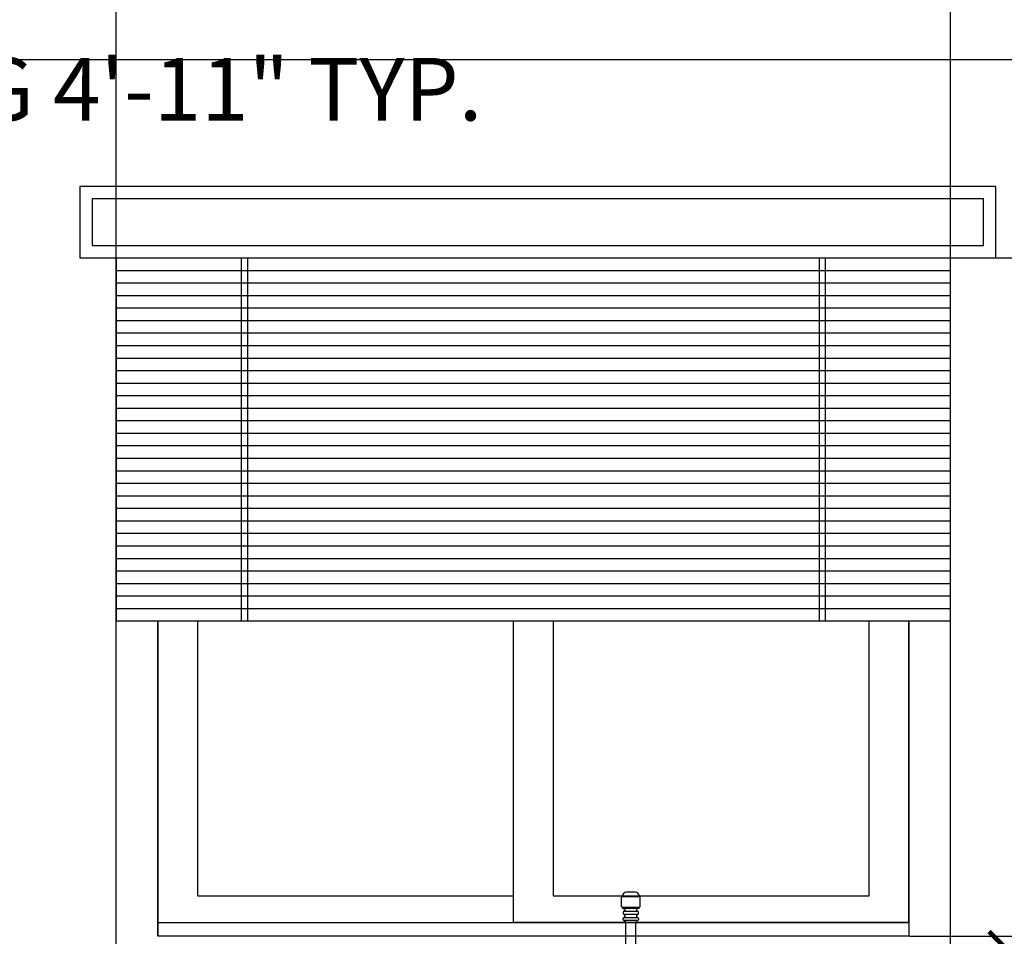
# Model space of a CAD drawing. Units: inches. Extents: x 2278 to 7495, y -71 to 1198.
# Tile 25 of 44: x 5007 to 5101, y 160 to 248. Entities that reach past the tile are written whole.
import ezdxf

# ---------------------------------------------------------------- set-up
doc = ezdxf.new("R2010")
doc.units = ezdxf.units.IN
doc.header["$MEASUREMENT"] = 0
doc.layers.add('A-ANNO-DIMS', color=2, linetype='Continuous', lineweight=18)
doc.layers.add('A-ELEV', color=7, linetype='Continuous', lineweight=25)
doc.styles.get("Standard").update_dxf_attribs({"font": 'arial.ttf'})
doc.dimstyles.get("Standard").update_dxf_attribs({"dimtxt": 6, "dimasz": 3, "dimexe": 0.18, "dimexo": 0.0625, "dimgap": 0.09, "dimtad": 0, "dimtih": 1, "dimtoh": 1, "dimdec": 0, "dimzin": 0, "dimdsep": 46, "dimlunit": 3, "dimtxsty": 'Standard', "dimblk": 'ARCHTICK', "dimcen": 0.09, "dimadec": 0, "dimazin": 0, "dimtfac": 1, "dimtdec": 0, "dimtofl": 0, "dimtmove": 0, "dimatfit": 3, "dimfxl": 1, "dimtolj": 1, "dimtzin": 0, "dimarcsym": 0})

# ---------------------------------------------------------------- blocks, each defined once
blk = doc.blocks.new('_ArchTick')
at = {"color": 0, "linetype": 'ByBlock', "const_width": 0.15}
blk.add_lwpolyline([(-0.5, -0.5), (0.5, 0.5)], dxfattribs=at)
blk = doc.blocks.new('*D57')
at = {"layer": 'A-ANNO-DIMS', "color": 0, "lineweight": -2, "transparency": 16777216}
for p, q in [((4874.676, 250.186), (4874.676, 241.236)), ((4933.558, 250.186), (4933.558, 241.236)), ((4874.676, 241.416), (4933.558, 241.416)), ((4933.558, 241.416), (4936.558, 241.416))]:
    blk.add_line(p, q, dxfattribs=at)
at = {"layer": 'Defpoints', "color": 0, "transparency": 16777216}
for p in [(4874.676, 250.248), (4933.558, 250.248), (4933.558, 241.416)]:
    blk.add_point(p, dxfattribs=at)
at = {"layer": 'A-ANNO-DIMS', "color": 0, "lineweight": -2, "transparency": 16777216, "xscale": 3, "yscale": 3, "zscale": 3, "rotation": 180}
blk.add_blockref('_ArchTick', (4874.676, 241.416), dxfattribs=at)
at = {"layer": 'A-ANNO-DIMS', "color": 0, "lineweight": -2, "transparency": 16777216, "xscale": 3, "yscale": 3, "zscale": 3}
blk.add_blockref('_ArchTick', (4933.558, 241.416), dxfattribs=at)
at = {"layer": 'A-ANNO-DIMS', "color": 0, "transparency": 16777216, "insert": (4995.776, 241.416), "char_height": 6, "attachment_point": 5}
blk.add_mtext('\\A1;PARAPET RAILING 4\'-11" TYP.', dxfattribs=at)
blk = doc.blocks.new('*D59')
at = {"layer": 'A-ANNO-DIMS', "color": 0, "lineweight": -2, "transparency": 16777216}
for p, q in [((5096.589, 159.183), (5101.564, 159.183)), ((5101.384, 159.183), (5101.384, 146.185)), ((5101.384, 126.799), (5101.384, 139.796)), ((5096.589, 126.799), (5101.564, 126.799))]:
    blk.add_line(p, q, dxfattribs=at)
at = {"layer": 'Defpoints', "color": 0, "transparency": 16777216}
for p in [(5096.527, 159.183), (5101.384, 159.183), (5096.527, 126.799)]:
    blk.add_point(p, dxfattribs=at)
at = {"layer": 'A-ANNO-DIMS', "color": 0, "lineweight": -2, "transparency": 16777216, "xscale": 3, "yscale": 3, "zscale": 3}
for p, rotation in [((5101.384, 159.183), 90), ((5101.384, 126.799), 270)]:
    blk.add_blockref('_ArchTick', p, dxfattribs=dict(at, rotation=rotation))
at = {"layer": 'A-ANNO-DIMS', "color": 0, "transparency": 16777216, "insert": (5101.384, 142.991), "char_height": 6, "attachment_point": 5}
blk.add_mtext('\\A1;ORNATE BALUSTER 2\'-8 1/2" TYP.', dxfattribs=at)
blk = doc.blocks.new('*D123')
at = {"layer": 'A-ANNO-DIMS', "color": 0, "lineweight": -2, "transparency": 16777216}
for p, q in [((4736.95, 340.157), (4736.95, -23.427)), ((5145.676, -1.81), (5145.676, -23.427)), ((4736.95, -23.247), (4923.929, -23.247)), ((5145.676, -23.247), (4958.697, -23.247))]:
    blk.add_line(p, q, dxfattribs=at)
at = {"layer": 'Defpoints', "color": 0, "transparency": 16777216}
for p in [(4736.95, 340.219), (5145.676, -1.747), (5145.676, -23.247)]:
    blk.add_point(p, dxfattribs=at)
at = {"layer": 'A-ANNO-DIMS', "color": 0, "lineweight": -2, "transparency": 16777216, "xscale": 3, "yscale": 3, "zscale": 3, "rotation": 180}
blk.add_blockref('_ArchTick', (4736.95, -23.247), dxfattribs=at)
at = {"layer": 'A-ANNO-DIMS', "color": 0, "lineweight": -2, "transparency": 16777216, "xscale": 3, "yscale": 3, "zscale": 3}
blk.add_blockref('_ArchTick', (5145.676, -23.247), dxfattribs=at)
at = {"layer": 'A-ANNO-DIMS', "color": 0, "transparency": 16777216, "insert": (4941.313, -23.247), "char_height": 6, "attachment_point": 5}
blk.add_mtext('\\A1;34\'-0 1/2"', dxfattribs=at)
blk = doc.blocks.new('*D129')
at = {"layer": 'A-ANNO-DIMS', "color": 0, "lineweight": -2, "transparency": 16777216}
for p, q in [((4970.676, 60.779), (4970.676, 361.899)), ((4970.676, 361.719), (4978.373, 361.719)), ((5016.176, 361.719), (5008.479, 361.719)), ((5016.176, 99.315), (5016.176, 361.899))]:
    blk.add_line(p, q, dxfattribs=at)
at = {"layer": 'Defpoints', "color": 0, "transparency": 16777216}
for p in [(5016.176, 361.719), (5016.176, 99.253), (4970.676, 60.717)]:
    blk.add_point(p, dxfattribs=at)
at = {"layer": 'A-ANNO-DIMS', "color": 0, "lineweight": -2, "transparency": 16777216, "xscale": 3, "yscale": 3, "zscale": 3, "rotation": 180}
blk.add_blockref('_ArchTick', (4970.676, 361.719), dxfattribs=at)
at = {"layer": 'A-ANNO-DIMS', "color": 0, "lineweight": -2, "transparency": 16777216, "xscale": 3, "yscale": 3, "zscale": 3}
blk.add_blockref('_ArchTick', (5016.176, 361.719), dxfattribs=at)
at = {"layer": 'A-ANNO-DIMS', "color": 0, "transparency": 16777216, "insert": (4993.426, 361.719), "char_height": 6, "attachment_point": 5}
blk.add_mtext('\\A1;3\'-9 1/2"', dxfattribs=at)
blk = doc.blocks.new('*D130')
at = {"layer": 'A-ANNO-DIMS', "color": 0, "lineweight": -2, "transparency": 16777216}
for p, q in [((5016.176, 99.315), (5016.176, 361.899)), ((5016.176, 361.719), (5048.095, 361.719)), ((5096.176, 361.719), (5064.257, 361.719)), ((5096.176, 99.315), (5096.176, 361.899))]:
    blk.add_line(p, q, dxfattribs=at)
at = {"layer": 'Defpoints', "color": 0, "transparency": 16777216}
for p in [(5096.176, 361.719), (5016.176, 99.253), (5096.176, 99.253)]:
    blk.add_point(p, dxfattribs=at)
at = {"layer": 'A-ANNO-DIMS', "color": 0, "lineweight": -2, "transparency": 16777216, "xscale": 3, "yscale": 3, "zscale": 3, "rotation": 180}
blk.add_blockref('_ArchTick', (5016.176, 361.719), dxfattribs=at)
at = {"layer": 'A-ANNO-DIMS', "color": 0, "lineweight": -2, "transparency": 16777216, "xscale": 3, "yscale": 3, "zscale": 3}
blk.add_blockref('_ArchTick', (5096.176, 361.719), dxfattribs=at)
at = {"layer": 'A-ANNO-DIMS', "color": 0, "transparency": 16777216, "insert": (5056.176, 361.719), "char_height": 6, "attachment_point": 5}
blk.add_mtext('\\A1;6\'-8"', dxfattribs=at)
blk = doc.blocks.new('*D131')
at = {"layer": 'A-ANNO-DIMS', "color": 0, "lineweight": -2, "transparency": 16777216}
for p, q in [((5096.176, 99.315), (5096.176, 361.899)), ((5096.176, 361.719), (5105.75, 361.719)), ((5145.676, 361.719), (5136.102, 361.719)), ((5145.676, 118.315), (5145.676, 361.899))]:
    blk.add_line(p, q, dxfattribs=at)
at = {"layer": 'Defpoints', "color": 0, "transparency": 16777216}
for p in [(5145.676, 361.719), (5145.676, 118.253), (5096.176, 99.253)]:
    blk.add_point(p, dxfattribs=at)
at = {"layer": 'A-ANNO-DIMS', "color": 0, "lineweight": -2, "transparency": 16777216, "xscale": 3, "yscale": 3, "zscale": 3, "rotation": 180}
blk.add_blockref('_ArchTick', (5096.176, 361.719), dxfattribs=at)
at = {"layer": 'A-ANNO-DIMS', "color": 0, "lineweight": -2, "transparency": 16777216, "xscale": 3, "yscale": 3, "zscale": 3}
blk.add_blockref('_ArchTick', (5145.676, 361.719), dxfattribs=at)
at = {"layer": 'A-ANNO-DIMS', "color": 0, "transparency": 16777216, "insert": (5120.926, 361.719), "char_height": 6, "attachment_point": 5}
blk.add_mtext('\\A1;4\'-1 1/2"', dxfattribs=at)
blk = doc.blocks.new('*D139')
at = {"layer": 'A-ANNO-DIMS', "color": 0, "lineweight": -2, "transparency": 16777216}
for p, q in [((5092.239, 160.253), (5167.754, 160.253)), ((5167.574, 160.253), (5167.574, 142.408)), ((5167.574, 118.253), (5167.574, 136.097)), ((5145.739, 118.253), (5167.754, 118.253))]:
    blk.add_line(p, q, dxfattribs=at)
at = {"layer": 'Defpoints', "color": 0, "transparency": 16777216}
for p in [(5092.176, 160.253), (5167.574, 160.253), (5145.676, 118.253)]:
    blk.add_point(p, dxfattribs=at)
at = {"layer": 'A-ANNO-DIMS', "color": 0, "lineweight": -2, "transparency": 16777216, "xscale": 3, "yscale": 3, "zscale": 3}
for p, rotation in [((5167.574, 160.253), 90), ((5167.574, 118.253), 270)]:
    blk.add_blockref('_ArchTick', p, dxfattribs=dict(at, rotation=rotation))
at = {"layer": 'A-ANNO-DIMS', "color": 0, "transparency": 16777216, "insert": (5167.574, 139.253), "char_height": 6, "attachment_point": 5}
blk.add_mtext('\\A1;3\'-6"', dxfattribs=at)
blk = doc.blocks.new('*D140')
at = {"layer": 'A-ANNO-DIMS', "color": 0, "lineweight": -2, "transparency": 16777216}
for p, q in [((5096.239, 225.253), (5167.754, 225.253)), ((5167.574, 225.253), (5167.574, 195.894)), ((5167.574, 160.253), (5167.574, 189.612)), ((5092.239, 160.253), (5167.754, 160.253))]:
    blk.add_line(p, q, dxfattribs=at)
at = {"layer": 'Defpoints', "color": 0, "transparency": 16777216}
for p in [(5096.176, 225.253), (5167.574, 225.253), (5092.176, 160.253)]:
    blk.add_point(p, dxfattribs=at)
at = {"layer": 'A-ANNO-DIMS', "color": 0, "lineweight": -2, "transparency": 16777216, "xscale": 3, "yscale": 3, "zscale": 3}
for p, rotation in [((5167.574, 225.253), 90), ((5167.574, 160.253), 270)]:
    blk.add_blockref('_ArchTick', p, dxfattribs=dict(at, rotation=rotation))
at = {"layer": 'A-ANNO-DIMS', "color": 0, "transparency": 16777216, "insert": (5167.574, 192.753), "char_height": 6, "attachment_point": 5}
blk.add_mtext('\\A1;5\'-5"', dxfattribs=at)
blk = doc.blocks.new('*D141')
at = {"layer": 'A-ANNO-DIMS', "color": 0, "lineweight": -2, "transparency": 16777216}
for p, q in [((5145.739, 244.253), (5167.754, 244.253)), ((5167.574, 244.253), (5167.574, 237.855)), ((5167.574, 225.253), (5167.574, 231.651)), ((5096.239, 225.253), (5167.754, 225.253))]:
    blk.add_line(p, q, dxfattribs=at)
at = {"layer": 'Defpoints', "color": 0, "transparency": 16777216}
for p in [(5145.676, 244.253), (5167.574, 244.253), (5096.176, 225.253)]:
    blk.add_point(p, dxfattribs=at)
at = {"layer": 'A-ANNO-DIMS', "color": 0, "lineweight": -2, "transparency": 16777216, "xscale": 3, "yscale": 3, "zscale": 3}
for p, rotation in [((5167.574, 244.253), 90), ((5167.574, 225.253), 270)]:
    blk.add_blockref('_ArchTick', p, dxfattribs=dict(at, rotation=rotation))
at = {"layer": 'A-ANNO-DIMS', "color": 0, "transparency": 16777216, "insert": (5167.574, 234.753), "char_height": 6, "attachment_point": 5}
blk.add_mtext('\\A1;1\'-7"', dxfattribs=at)

msp = doc.modelspace()

# ---------------------------------------------------------------- linework, layer by layer
at = {"layer": 'A-ELEV'}
for p, q in [((4874.676, 244.253), (5145.676, 244.253)), ((5016.176, 225.253), (5096.176, 225.253)), ((5016.176, 225.253), (5016.176, 190.453)), ((5028.176, 225.253), (5028.176, 190.453)), ((5028.176, 225.253), (5028.176, 191.653)), ((5028.176, 225.253), (5028.176, 191.653)), ((5028.176, 225.253), (5028.176, 191.653)), ((5028.776, 225.253), (5028.776, 190.453)), ((5028.776, 225.253), (5028.776, 191.653)), ((5028.776, 225.253), (5028.776, 191.653)), ((5028.776, 225.253), (5028.776, 191.653)), ((5083.576, 225.253), (5083.576, 190.453)), ((5083.576, 225.253), (5083.576, 191.653)), ((5083.576, 225.253), (5083.576, 191.653)), ((5083.576, 225.253), (5083.576, 191.653)), ((5084.176, 225.253), (5084.176, 190.453)), ((5084.176, 225.253), (5084.176, 191.653)), ((5084.176, 225.253), (5084.176, 191.653)), ((5084.176, 225.253), (5084.176, 191.653)), ((5096.176, 190.453), (5096.176, 225.253)), ((5016.176, 224.053), (5096.176, 224.053)), ((5016.176, 222.853), (5096.176, 222.853)), ((5016.176, 221.653), (5096.176, 221.653)), ((5016.176, 220.453), (5096.176, 220.453)), ((5016.176, 219.253), (5096.176, 219.253)), ((5016.176, 218.053), (5096.176, 218.053)), ((5016.176, 216.853), (5096.176, 216.853)), ((5016.176, 215.653), (5096.176, 215.653)), ((5016.176, 214.453), (5096.176, 214.453)), ((5016.176, 213.253), (5096.176, 213.253)), ((5016.176, 212.053), (5096.176, 212.053)), ((5016.176, 210.853), (5096.176, 210.853)), ((5016.176, 209.653), (5096.176, 209.653)), ((5016.176, 208.453), (5096.176, 208.453)), ((5016.176, 207.253), (5096.176, 207.253)), ((5016.176, 206.053), (5096.176, 206.053)), ((5016.176, 204.853), (5096.176, 204.853)), ((5016.176, 203.653), (5096.176, 203.653)), ((5016.176, 202.453), (5096.176, 202.453)), ((5016.176, 201.253), (5096.176, 201.253)), ((5016.176, 200.053), (5096.176, 200.053)), ((5016.176, 198.853), (5096.176, 198.853)), ((5016.176, 197.653), (5096.176, 197.653)), ((5016.176, 196.453), (5096.176, 196.453)), ((5016.176, 195.253), (5096.176, 195.253)), ((5016.176, 194.053), (5096.176, 194.053)), ((5016.176, 192.853), (5096.176, 192.853)), ((5016.176, 191.653), (5096.176, 191.653)), ((5016.176, 190.453), (5096.176, 190.453)), ((5020.176, 160.253), (5020.176, 190.453)), ((5020.176, 160.253), (5020.176, 190.453)), ((5020.176, 190.453), (5020.176, 160.253)), ((5020.176, 190.453), (5020.176, 161.539)), ((5020.176, 190.453), (5020.176, 161.539)), ((5023.966, 190.453), (5023.966, 164.11)), ((5023.966, 190.453), (5023.966, 164.11)), ((5054.282, 161.539), (5054.282, 190.453)), ((5054.282, 161.539), (5054.282, 190.453)), ((5058.071, 190.453), (5058.071, 164.11)), ((5058.071, 190.453), (5058.071, 164.11)), ((5088.387, 164.11), (5088.387, 190.453)), ((5088.387, 164.11), (5088.387, 190.453)), ((5092.176, 190.453), (5092.176, 161.539)), ((5092.176, 190.453), (5092.176, 161.539)), ((5092.176, 190.453), (5092.176, 160.253)), ((5092.176, 190.453), (5092.176, 160.253)), ((5092.176, 190.453), (5092.176, 160.253)), ((5092.176, 161.539), (5092.176, 190.453)), ((5065.988, 164.449), (5065.066, 164.449)), ((5023.966, 164.11), (5054.282, 164.11)), ((5023.966, 164.11), (5054.282, 164.11)), ((5058.071, 164.11), (5088.387, 164.11)), ((5058.071, 164.11), (5088.387, 164.11)), ((5064.641, 163.092), (5064.641, 163.965)), ((5064.722, 164.046), (5066.332, 164.046)), ((5064.737, 164.122), (5064.737, 164.046)), ((5066.318, 164.122), (5066.318, 164.046)), ((5066.414, 163.092), (5066.414, 163.965)), ((5064.722, 163.01), (5066.332, 163.01)), ((5064.737, 162.934), (5064.737, 163.01)), ((5064.737, 162.934), (5064.962, 162.837)), ((5064.737, 162.934), (5066.318, 162.934)), ((5064.794, 162.533), (5064.794, 162.416)), ((5064.876, 162.615), (5064.962, 162.711)), ((5066.179, 162.615), (5064.876, 162.615)), ((5066.318, 162.934), (5066.093, 162.837)), ((5066.179, 162.615), (5066.093, 162.711)), ((5066.261, 162.416), (5066.261, 162.533)), ((5066.318, 162.934), (5066.318, 163.01)), ((5020.176, 161.539), (5092.176, 161.539)), ((5020.176, 161.539), (5092.176, 161.539)), ((5092.176, 161.539), (5054.282, 161.539)), ((5064.794, 161.816), (5064.794, 161.934)), ((5064.876, 162.334), (5064.962, 162.238)), ((5064.876, 162.334), (5066.179, 162.334)), ((5064.876, 162.015), (5064.962, 162.112)), ((5064.876, 162.015), (5066.179, 162.015)), ((5064.876, 161.735), (5065.009, 161.64)), ((5066.179, 161.735), (5064.876, 161.735)), ((5065.039, 147.642), (5065.039, 161.577)), ((5066.016, 147.642), (5066.016, 161.577)), ((5066.179, 161.735), (5066.046, 161.64)), ((5066.179, 162.334), (5066.093, 162.238)), ((5066.179, 162.015), (5066.093, 162.112)), ((5066.261, 161.934), (5066.261, 161.816)), ((5092.176, 160.253), (5020.176, 160.253)), ((5092.176, 160.253), (5020.176, 160.253)), ((5092.176, 160.253), (5020.176, 160.253)), ((5020.176, 160.253), (5020.176, 160.253))]:
    msp.add_line(p, q, dxfattribs=at)
for points in [[(5012.694, 225.253), (5100.529, 225.253), (5100.529, 232.097), (5012.694, 232.097)], [(5013.894, 226.453), (5099.329, 226.453), (5099.329, 230.897), (5013.894, 230.897)]]:
    msp.add_lwpolyline(points, close=True, dxfattribs=at)
for centre, radius, start, end in [((5065.089, 164.097), 0.352, 93.62058, 175.89193), ((5065.966, 164.097), 0.352, 4.10807, 86.37942), ((5064.722, 163.965), 0.0815, 90, 180), ((5066.332, 163.965), 0.0815, 0, 90), ((5064.722, 163.092), 0.0815, 180, 270), ((5064.876, 162.533), 0.0815, 90, 180), ((5064.876, 162.416), 0.0815, 180, 270), ((5064.91, 162.774), 0.0815, 309.328, 50.672), ((5066.145, 162.774), 0.0815, 129.328, 230.672), ((5066.179, 162.533), 0.0815, 0, 90), ((5066.179, 162.416), 0.0815, 270, 360), ((5066.332, 163.092), 0.0815, 270, 0), ((5064.876, 161.934), 0.0815, 90, 180), ((5064.876, 161.816), 0.0815, 180, 270), ((5064.91, 162.175), 0.0815, 309.328, 50.672), ((5064.957, 161.577), 0.0815, 0, 50.672), ((5066.098, 161.577), 0.0815, 129.328, 180), ((5066.145, 162.175), 0.0815, 129.328, 230.672), ((5066.179, 161.934), 0.0815, 0, 90), ((5066.179, 161.816), 0.0815, 270, 360)]:
    msp.add_arc(centre, radius, start, end, dxfattribs=at)

# ---------------------------------------------------------------- dimensions: what is measured, and where the dimension line sits
at = {"layer": 'A-ANNO-DIMS'}
for base, p1, p2, picture, middle in [((5016.176, 361.719), (4970.676, 60.717), (5016.176, 99.253), '*D129', (4993.426, 361.719)), ((5145.676, 361.719), (5096.176, 99.253), (5145.676, 118.253), '*D131', (5120.926, 361.719)), ((5096.176, 361.719), (5016.176, 99.253), (5096.176, 99.253), '*D130', (5056.176, 361.719)), ((5145.676, -23.247), (4736.95, 340.219), (5145.676, -1.747), '*D123', (4941.313, -23.247))]:
    dim = msp.add_linear_dim(base=base, p1=p1, p2=p2, dimstyle='Standard', override={"dimdec": 1, "dimlfac": 1, "dimrnd": 0, "dimzin": 1, "dimdsep": 46, "dimlunit": 4, "dimfrac": 2}, dxfattribs=at)
    dim.commit()
    dim.dimension.update_dxf_attribs({"geometry": picture, "text_midpoint": middle})
dim = msp.add_linear_dim(base=(4933.558, 241.416), p1=(4874.676, 250.248), p2=(4933.558, 250.248), text='PARAPET RAILING <> TYP.', dimstyle='Standard', override={"dimdec": 1, "dimrnd": 0, "dimzin": 1, "dimlunit": 4, "dimfrac": 2}, dxfattribs=at)
dim.commit()
dim.dimension.update_dxf_attribs({"geometry": '*D57', "text_midpoint": (4995.776, 241.416)})
for base, p1, p2, picture, middle in [((5167.574, 244.253), (5096.176, 225.253), (5145.676, 244.253), '*D141', (5167.574, 234.753)), ((5167.574, 225.253), (5092.176, 160.253), (5096.176, 225.253), '*D140', (5167.574, 192.753)), ((5167.574, 160.253), (5145.676, 118.253), (5092.176, 160.253), '*D139', (5167.574, 139.253))]:
    dim = msp.add_linear_dim(base=base, p1=p1, p2=p2, angle=90, dimstyle='Standard', override={"dimdec": 1, "dimlfac": 1, "dimrnd": 0, "dimzin": 1, "dimdsep": 46, "dimlunit": 4, "dimfrac": 2}, dxfattribs=at)
    dim.commit()
    dim.dimension.update_dxf_attribs({"geometry": picture, "text_midpoint": middle})
dim = msp.add_linear_dim(base=(5101.384, 159.183), p1=(5096.527, 126.799), p2=(5096.527, 159.183), angle=90, text='ORNATE BALUSTER <> TYP.', dimstyle='Standard', override={"dimdec": 1, "dimrnd": 0, "dimzin": 1, "dimlunit": 4, "dimfrac": 2}, dxfattribs=at)
dim.commit()
dim.dimension.update_dxf_attribs({"geometry": '*D59', "text_midpoint": (5101.384, 142.991)})

doc.saveas('drawing.dxf')
